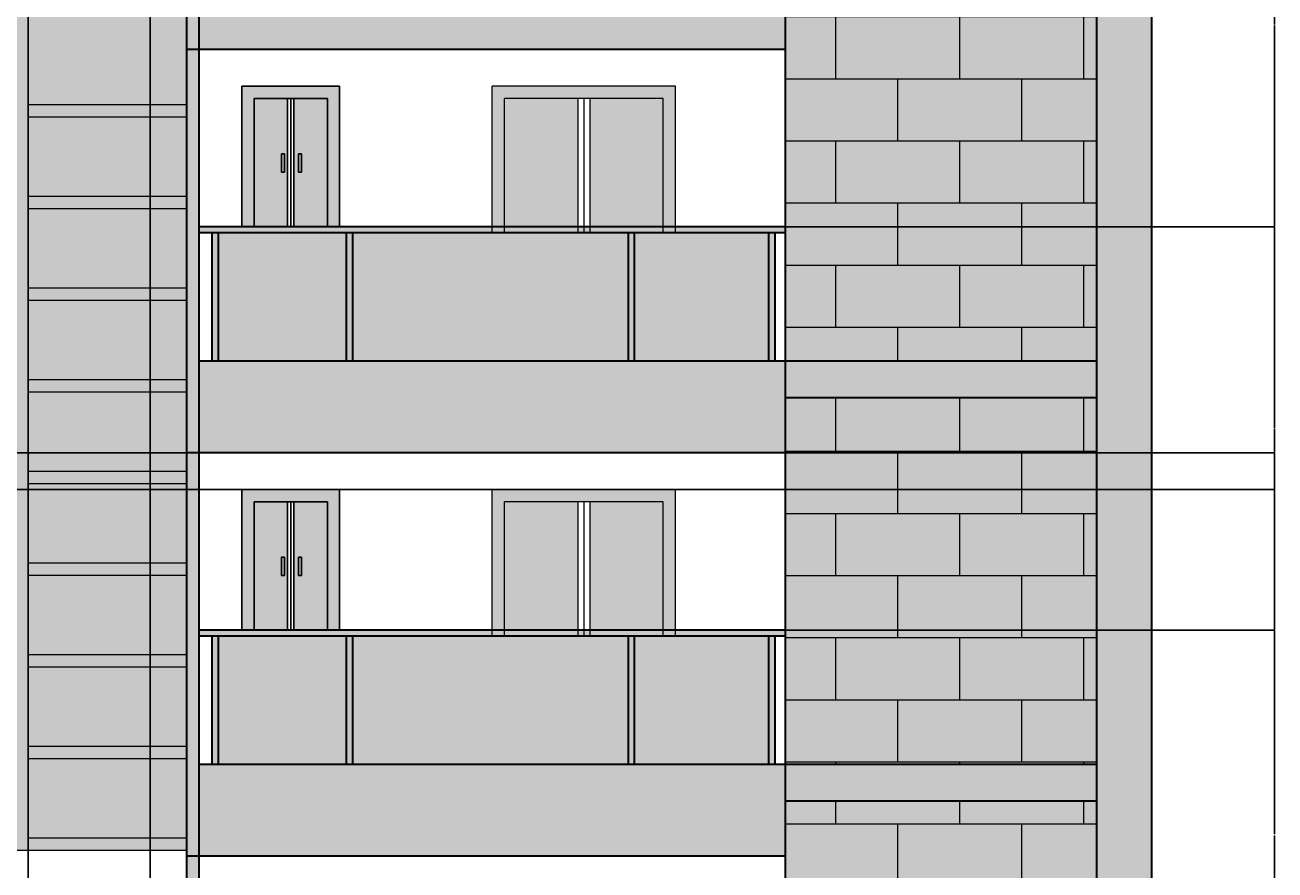
# Model space of a CAD drawing. Units: inches. Extents: x 2794 to 3619, y 522 to 1397.
# Tile 6 of 10: x 3209 to 3619, y 696 to 973. Entities that reach past the tile are written whole.
import ezdxf

# ---------------------------------------------------------------- set-up
doc = ezdxf.new("R2010")
doc.units = ezdxf.units.IN
for name, color, linetype, lineweight in [('A-ANNO-DIMS', 2, 'Continuous', 18), ('A-DOOR', 3, 'Continuous', 25), ('A-ELEV', 7, 'Continuous', 35), ('A-ELEV-PATT', 8, 'Continuous', 13), ('A-GLAZ', 4, 'Continuous', 18)]:
    doc.layers.add(name, color=color, linetype=linetype, lineweight=lineweight)
doc.styles.get("Standard").update_dxf_attribs({"font": 'arial.ttf'})
doc.dimstyles.get("Standard").update_dxf_attribs({"dimtxt": 0.18, "dimasz": 0.18, "dimexe": 0.18, "dimexo": 0.0625, "dimgap": 0.09, "dimtad": 0, "dimtih": 1, "dimtoh": 1, "dimdec": 4, "dimzin": 0, "dimdsep": 46, "dimtxsty": 'Standard', "dimcen": 0.09, "dimadec": 0, "dimazin": 0, "dimtfac": 1, "dimtdec": 4, "dimtofl": 0, "dimtmove": 0, "dimatfit": 3, "dimfxl": 1, "dimtolj": 1, "dimtzin": 0, "dimarcsym": 0})

# ---------------------------------------------------------------- blocks, each defined once
blk = doc.blocks.new('WIN-1500')
at = {"transparency": 33554646}
h = blk.add_hatch(color=256, dxfattribs=at)
h.dxf.hatch_style = 1
h.paths.add_polyline_path([(60, 48), (0, 48), (0, 2), (4, 2), (4, 44), (56, 44), (56, 2), (60, 2)])
at = {"transparency": 33554687}
h = blk.add_hatch(color=256, dxfattribs=at)
h.dxf.hatch_style = 1
h.set_gradient(color1=(248, 246, 176), color2=(74, 13, 14), name='INVCYLINDER')
h.paths.add_polyline_path([(56, 44), (32, 44), (32, 2), (56, 2)])
h.paths.add_polyline_path([(28, 44), (4, 44), (4, 2), (28, 2)])
for p, q in [((0, 0), (0, 48)), ((60, 48), (0, 48)), ((60, 0), (60, 48)), ((56, 44), (4, 44)), ((4, 0), (4, 44)), ((28, 44), (28, 0)), ((30, 44), (30, 0)), ((32, 44), (32, 0)), ((56, 0), (56, 44))]:
    blk.add_line(p, q)
blk = doc.blocks.new('DOOR-BALCONY-DBL')
at = {"transparency": 33554628}
h = blk.add_hatch(color=256, dxfattribs=at)
h.dxf.hatch_style = 1
h.paths.add_polyline_path([(4, 42), (28, 42), (28, 0), (32, 0), (32, 46), (0, 46), (0, 0), (4, 0)])
at = {"transparency": 33554646}
h = blk.add_hatch(color=256, dxfattribs=at)
h.dxf.hatch_style = 1
h.set_gradient(color1=(255, 255, 255), color2=(147, 149, 152), name='INVCYLINDER')
h.paths.add_polyline_path([(15, 42), (4, 42), (4, 0), (15, 0)])
h = blk.add_hatch(color=256, dxfattribs=at)
h.dxf.hatch_style = 1
h.set_gradient(color1=(255, 255, 255), color2=(147, 149, 152), name='INVCYLINDER')
h.paths.add_polyline_path([(28, 42), (17, 42), (17, 0), (28, 0)])
for p, q in [((0, 0), (0, 46)), ((0, 46), (32, 46)), ((4, 46), (28, 46)), ((32, 0), (32, 46)), ((4, 0), (4, 42)), ((4, 42), (28, 42)), ((15, 0), (15, 42)), ((16, 0), (16, 42)), ((17, 0), (17, 42)), ((28, 0), (28, 42))]:
    blk.add_line(p, q)
for points in [[(12.99, 23.83), (13.93, 23.83), (13.93, 17.87), (12.99, 17.87)], [(18.59, 23.83), (19.53, 23.83), (19.53, 17.87), (18.59, 17.87)]]:
    blk.add_lwpolyline(points, close=True)
blk = doc.blocks.new('*D19')
at = {"layer": 'A-ANNO-DIMS', "color": 0, "lineweight": -2, "transparency": 16777216}
for p, q in [((3458.33, 774.64), (3618.55, 774.64)), ((3618.37, 774.46), (3618.37, 707.82)), ((3618.37, 640.82), (3618.37, 707.45)), ((3458.33, 640.64), (3618.55, 640.64))]:
    blk.add_line(p, q, dxfattribs=at)
at = {"layer": 'A-ANNO-DIMS', "color": 0, "transparency": 16777216}
for points in [[(3618.34, 774.46), (3618.4, 774.46), (3618.37, 774.64)], [(3618.34, 640.82), (3618.4, 640.82), (3618.37, 640.64)]]:
    blk.add_solid(points, dxfattribs=at)
at = {"layer": 'Defpoints', "color": 0, "transparency": 16777216}
for p in [(3458.27, 774.64), (3618.37, 774.64), (3458.27, 640.64)]:
    blk.add_point(p, dxfattribs=at)
at = {"layer": 'A-ANNO-DIMS', "color": 0, "transparency": 16777216, "insert": (3618.37, 707.64), "char_height": 0.18, "attachment_point": 5}
blk.add_mtext('\\A1;134', dxfattribs=at)
blk = doc.blocks.new('*D20')
at = {"layer": 'A-ANNO-DIMS', "color": 0, "lineweight": -2, "transparency": 16777216}
for p, q in [((3458.33, 906.64), (3618.55, 906.64)), ((3618.37, 906.46), (3618.37, 840.82)), ((3618.37, 774.82), (3618.37, 840.45)), ((3458.33, 774.64), (3618.55, 774.64))]:
    blk.add_line(p, q, dxfattribs=at)
at = {"layer": 'A-ANNO-DIMS', "color": 0, "transparency": 16777216}
for points in [[(3618.34, 906.46), (3618.4, 906.46), (3618.37, 906.64)], [(3618.34, 774.82), (3618.4, 774.82), (3618.37, 774.64)]]:
    blk.add_solid(points, dxfattribs=at)
at = {"layer": 'Defpoints', "color": 0, "transparency": 16777216}
for p in [(3458.27, 906.64), (3618.37, 906.64), (3458.27, 774.64)]:
    blk.add_point(p, dxfattribs=at)
at = {"layer": 'A-ANNO-DIMS', "color": 0, "transparency": 16777216, "insert": (3618.37, 840.64), "char_height": 0.18, "attachment_point": 5}
blk.add_mtext('\\A1;132', dxfattribs=at)
blk = doc.blocks.new('*D21')
at = {"layer": 'A-ANNO-DIMS', "color": 0, "lineweight": -2, "transparency": 16777216}
for p, q in [((3458.33, 1038.64), (3618.55, 1038.64)), ((3618.37, 1038.46), (3618.37, 972.82)), ((3618.37, 906.82), (3618.37, 972.45)), ((3458.33, 906.64), (3618.55, 906.64))]:
    blk.add_line(p, q, dxfattribs=at)
at = {"layer": 'A-ANNO-DIMS', "color": 0, "transparency": 16777216}
for points in [[(3618.34, 1038.46), (3618.4, 1038.46), (3618.37, 1038.64)], [(3618.34, 906.82), (3618.4, 906.82), (3618.37, 906.64)]]:
    blk.add_solid(points, dxfattribs=at)
at = {"layer": 'Defpoints', "color": 0, "transparency": 16777216}
for p in [(3458.27, 1038.64), (3618.37, 1038.64), (3458.27, 906.64)]:
    blk.add_point(p, dxfattribs=at)
at = {"layer": 'A-ANNO-DIMS', "color": 0, "transparency": 16777216, "insert": (3618.37, 972.64), "char_height": 0.18, "attachment_point": 5}
blk.add_mtext('\\A1;132', dxfattribs=at)
blk = doc.blocks.new('*D43')
at = {"layer": 'A-ANNO-DIMS', "color": 0, "lineweight": -2, "transparency": 16777216}
for p, q in [((3150.33, 832.64), (3618.55, 832.64)), ((3618.37, 832.46), (3618.37, 826.82)), ((3618.37, 820.82), (3618.37, 826.45)), ((3132.33, 820.64), (3618.55, 820.64))]:
    blk.add_line(p, q, dxfattribs=at)
at = {"layer": 'A-ANNO-DIMS', "color": 0, "transparency": 16777216}
for points in [[(3618.34, 832.46), (3618.4, 832.46), (3618.37, 832.64)], [(3618.34, 820.82), (3618.4, 820.82), (3618.37, 820.64)]]:
    blk.add_solid(points, dxfattribs=at)
at = {"layer": 'Defpoints', "color": 0, "transparency": 16777216}
for p in [(3150.27, 832.64), (3618.37, 832.64), (3132.27, 820.64)]:
    blk.add_point(p, dxfattribs=at)
at = {"layer": 'A-ANNO-DIMS', "color": 0, "transparency": 16777216, "insert": (3618.37, 826.64), "char_height": 0.18, "attachment_point": 5}
blk.add_mtext('\\A1;12', dxfattribs=at)
blk = doc.blocks.new('*D51')
at = {"layer": 'A-ANNO-DIMS', "color": 0, "lineweight": -2, "transparency": 16777216}
for p, q in [((3206.27, 1254.57), (3206.27, 522.36)), ((3210.27, 1254.57), (3210.27, 522.36)), ((3206.45, 522.54), (3208.11, 522.54)), ((3210.09, 522.54), (3208.42, 522.54))]:
    blk.add_line(p, q, dxfattribs=at)
at = {"layer": 'A-ANNO-DIMS', "color": 0, "transparency": 16777216}
for points in [[(3206.45, 522.57), (3206.45, 522.51), (3206.27, 522.54)], [(3210.09, 522.57), (3210.09, 522.51), (3210.27, 522.54)]]:
    blk.add_solid(points, dxfattribs=at)
at = {"layer": 'Defpoints', "color": 0, "transparency": 16777216}
for p in [(3206.27, 1254.64), (3210.27, 1254.64), (3210.27, 522.54)]:
    blk.add_point(p, dxfattribs=at)
at = {"layer": 'A-ANNO-DIMS', "color": 0, "transparency": 16777216, "insert": (3208.27, 522.54), "char_height": 0.18, "attachment_point": 5}
blk.add_mtext('\\A1;4', dxfattribs=at)
blk = doc.blocks.new('*D52')
at = {"layer": 'A-ANNO-DIMS', "color": 0, "lineweight": -2, "transparency": 16777216}
for p, q in [((3210.27, 1254.57), (3210.27, 522.36)), ((3262.27, 1254.57), (3262.27, 522.36)), ((3210.45, 522.54), (3236.05, 522.54)), ((3262.09, 522.54), (3236.48, 522.54))]:
    blk.add_line(p, q, dxfattribs=at)
at = {"layer": 'A-ANNO-DIMS', "color": 0, "transparency": 16777216}
for points in [[(3210.45, 522.57), (3210.45, 522.51), (3210.27, 522.54)], [(3262.09, 522.57), (3262.09, 522.51), (3262.27, 522.54)]]:
    blk.add_solid(points, dxfattribs=at)
at = {"layer": 'Defpoints', "color": 0, "transparency": 16777216}
for p in [(3210.27, 1254.64), (3262.27, 1254.64), (3262.27, 522.54)]:
    blk.add_point(p, dxfattribs=at)
at = {"layer": 'A-ANNO-DIMS', "color": 0, "transparency": 16777216, "insert": (3236.27, 522.54), "char_height": 0.18, "attachment_point": 5}
blk.add_mtext('\\A1;52', dxfattribs=at)
blk = doc.blocks.new('*D56')
at = {"layer": 'A-ANNO-DIMS', "color": 0, "lineweight": -2, "transparency": 16777216}
for p, q in [((3162.27, 664.7), (3162.27, 1396.92)), ((3162.45, 1396.74), (3206.05, 1396.74)), ((3250.09, 1396.74), (3206.49, 1396.74)), ((3250.27, 664.7), (3250.27, 1396.92))]:
    blk.add_line(p, q, dxfattribs=at)
at = {"layer": 'A-ANNO-DIMS', "color": 0, "transparency": 16777216}
for points in [[(3162.45, 1396.77), (3162.45, 1396.71), (3162.27, 1396.74)], [(3250.09, 1396.77), (3250.09, 1396.71), (3250.27, 1396.74)]]:
    blk.add_solid(points, dxfattribs=at)
at = {"layer": 'Defpoints', "color": 0, "transparency": 16777216}
for p in [(3250.27, 1396.74), (3162.27, 664.64), (3250.27, 664.64)]:
    blk.add_point(p, dxfattribs=at)
at = {"layer": 'A-ANNO-DIMS', "color": 0, "transparency": 16777216, "insert": (3206.27, 1396.74), "char_height": 0.18, "attachment_point": 5}
blk.add_mtext('\\A1;88', dxfattribs=at)

msp = doc.modelspace()

# ---------------------------------------------------------------- hatches: boundary and pattern name
at = {"layer": 'A-ELEV-PATT', "transparency": 33554687}
h = msp.add_hatch(color=256, dxfattribs=at)
h.dxf.hatch_style = 1
h.paths.add_polyline_path([(3262.2659, 1350.6351), (3150.2659, 1350.6351), (3150.2659, 1279.0155, -0.68639605), (3262.2659, 1279.0155)])
h.paths.add_polyline_path([(3210.2659, 1314.1121), (3210.2659, 1258.6351), (3262.2659, 1258.6351, 0.39146256)])
h.paths.add_polyline_path([(3206.2659, 1314.2551, 0.41222069), (3150.2659, 1258.6351), (3206.2659, 1258.6351)])
h.paths.add_polyline_path([(3262.2659, 1254.6351), (3210.2659, 1254.6351), (3210.2659, 1216.6351), (3262.2659, 1216.6351)])
h.paths.add_polyline_path([(3206.2659, 1254.6351), (3150.2659, 1254.6351), (3150.2659, 1216.6351), (3206.2659, 1216.6351)])
h.paths.add_polyline_path([(3262.2659, 1212.6351), (3210.2659, 1212.6351), (3210.2659, 1186.6351), (3262.2659, 1186.6351)])
h.paths.add_polyline_path([(3206.2659, 1212.6351), (3150.2659, 1212.6351), (3150.2659, 1186.6351), (3206.2659, 1186.6351)])
h.paths.add_polyline_path([(3206.2659, 1182.6351), (3150.2659, 1182.6351), (3150.2659, 1156.6351), (3206.2659, 1156.6351)])
h.paths.add_polyline_path([(3262.2659, 1182.6351), (3210.2659, 1182.6351), (3210.2659, 1156.6351), (3262.2659, 1156.6351)])
h.paths.add_polyline_path([(3262.2659, 1152.6351), (3210.2659, 1152.6351), (3210.2659, 1126.6351), (3262.2659, 1126.6351)])
h.paths.add_polyline_path([(3206.2659, 1152.6351), (3150.2659, 1152.6351), (3150.2659, 1126.6351), (3206.2659, 1126.6351)])
h.paths.add_polyline_path([(3262.2659, 1122.6351), (3210.2659, 1122.6351), (3210.2659, 1096.6351), (3262.2659, 1096.6351)])
h.paths.add_polyline_path([(3206.2659, 1122.6351), (3150.2659, 1122.6351), (3150.2659, 1096.6351), (3206.2659, 1096.6351)])
h.paths.add_polyline_path([(3206.2659, 1092.6351), (3150.2659, 1092.6351), (3150.2659, 1066.6351), (3206.2659, 1066.6351)])
h.paths.add_polyline_path([(3262.2659, 1092.6351), (3210.2659, 1092.6351), (3210.2659, 1066.6351), (3262.2659, 1066.6351)])
h.paths.add_polyline_path([(3262.2659, 1062.6351), (3210.2659, 1062.6351), (3210.2659, 1036.6351), (3262.2659, 1036.6351)])
h.paths.add_polyline_path([(3206.2659, 1062.6351), (3150.2659, 1062.6351), (3150.2659, 1036.6351), (3206.2659, 1036.6351)])
h.paths.add_polyline_path([(3206.2659, 1032.6351), (3150.2659, 1032.6351), (3150.2659, 1006.6351), (3206.2659, 1006.6351)])
h.paths.add_polyline_path([(3262.2659, 1032.6351), (3210.2659, 1032.6351), (3210.2659, 1006.6351), (3262.2659, 1006.6351)])
h.paths.add_polyline_path([(3262.2659, 1002.6351), (3210.2659, 1002.6351), (3210.2659, 976.6351), (3262.2659, 976.6351)])
h.paths.add_polyline_path([(3206.2659, 1002.6351), (3150.2659, 1002.6351), (3150.2659, 976.6351), (3206.2659, 976.6351)])
h.paths.add_polyline_path([(3206.2659, 972.6351), (3150.2659, 972.6351), (3150.2659, 946.6351), (3206.2659, 946.6351)])
h.paths.add_polyline_path([(3206.2659, 942.6351), (3150.2659, 942.6351), (3150.2659, 916.6351), (3206.2659, 916.6351)])
h.paths.add_polyline_path([(3262.2659, 942.6351), (3210.2659, 942.6351), (3210.2659, 916.6351), (3262.2659, 916.6351)])
h.paths.add_polyline_path([(3262.2659, 972.6351), (3210.2659, 972.6351), (3210.2659, 946.6351), (3262.2659, 946.6351)])
h.paths.add_polyline_path([(3262.2659, 912.6351), (3210.2659, 912.6351), (3210.2659, 886.6351), (3262.2659, 886.6351)])
h.paths.add_polyline_path([(3206.2659, 912.6351), (3150.2659, 912.6351), (3150.2659, 886.6351), (3206.2659, 886.6351)])
h.paths.add_polyline_path([(3206.2659, 882.6351), (3150.2659, 882.6351), (3150.2659, 856.6351), (3206.2659, 856.6351)])
h.paths.add_polyline_path([(3262.2659, 882.6351), (3210.2659, 882.6351), (3210.2659, 856.6351), (3262.2659, 856.6351)])
h.paths.add_polyline_path([(3262.2659, 852.6351), (3210.2659, 852.6351), (3210.2659, 826.6351), (3262.2659, 826.6351)])
h.paths.add_polyline_path([(3206.2659, 852.6351), (3150.2659, 852.6351), (3150.2659, 826.6351), (3206.2659, 826.6351)])
h.paths.add_polyline_path([(3206.2659, 822.6351), (3150.2659, 822.6351), (3150.2659, 796.6351), (3206.2659, 796.6351)])
h.paths.add_polyline_path([(3262.2659, 822.6351), (3210.2659, 822.6351), (3210.2659, 796.6351), (3262.2659, 796.6351)])
h.paths.add_polyline_path([(3262.2659, 792.6351), (3210.2659, 792.6351), (3210.2659, 766.6351), (3262.2659, 766.6351)])
h.paths.add_polyline_path([(3206.2659, 792.6351), (3150.2659, 792.6351), (3150.2659, 766.6351), (3206.2659, 766.6351)])
h.paths.add_polyline_path([(3206.2659, 762.6351), (3150.2659, 762.6351), (3150.2659, 736.6351), (3206.2659, 736.6351)])
h.paths.add_polyline_path([(3206.2659, 732.6351), (3150.2659, 732.6351), (3150.2659, 706.6351), (3206.2659, 706.6351)])
h.paths.add_polyline_path([(3262.2659, 732.6351), (3210.2659, 732.6351), (3210.2659, 706.6351), (3262.2659, 706.6351)])
h.paths.add_polyline_path([(3262.2659, 762.6351), (3210.2659, 762.6351), (3210.2659, 736.6351), (3262.2659, 736.6351)])
h = msp.add_hatch(color=256, dxfattribs=at)
h.dxf.hatch_style = 1
h.paths.add_polyline_path([(3150.2659, 1257.8725, -0.00340445), (3150.2659, 1258.6351), (3146.2659, 1258.6351), (3146.2659, 1228.6351), (3150.2659, 1228.6351)])
h.paths.add_polyline_path([(3262.2659, 1258.6351), (3210.2659, 1258.6351), (3210.2659, 1314.1121, 0.01787385), (3206.2659, 1314.2551), (3206.2659, 1258.6351), (3150.2659, 1258.6351), (3150.2659, 1254.6351), (3206.2659, 1254.6351), (3206.2659, 1216.6351), (3150.2659, 1216.6351), (3150.2659, 1212.6351), (3206.2659, 1212.6351), (3206.2659, 1186.6351), (3150.2659, 1186.6351), (3150.2659, 1182.6351), (3206.2659, 1182.6351), (3206.2659, 1156.6351), (3150.2659, 1156.6351), (3150.2659, 1152.6351), (3206.2659, 1152.6351), (3206.2659, 1126.6351), (3150.2659, 1126.6351), (3150.2659, 1122.6351), (3206.2659, 1122.6351), (3206.2659, 1096.6351), (3150.2659, 1096.6351), (3150.2659, 1092.6351), (3206.2659, 1092.6351), (3206.2659, 1066.6351), (3150.2659, 1066.6351), (3150.2659, 1062.6351), (3206.2659, 1062.6351), (3206.2659, 1036.6351), (3150.2659, 1036.6351), (3150.2659, 1032.6351), (3206.2659, 1032.6351), (3206.2659, 1006.6351), (3150.2659, 1006.6351), (3150.2659, 1002.6351), (3206.2659, 1002.6351), (3206.2659, 976.6351), (3150.2659, 976.6351), (3150.2659, 972.6351), (3206.2659, 972.6351), (3206.2659, 946.6351), (3150.2659, 946.6351), (3150.2659, 942.6351), (3206.2659, 942.6351), (3206.2659, 916.6351), (3150.2659, 916.6351), (3150.2659, 912.6351), (3206.2659, 912.6351), (3206.2659, 886.6351), (3150.2659, 886.6351), (3150.2659, 882.6351), (3206.2659, 882.6351), (3206.2659, 856.6351), (3150.2659, 856.6351), (3150.2659, 852.6351), (3206.2659, 852.6351), (3206.2659, 826.6351), (3150.2659, 826.6351), (3150.2659, 822.6351), (3206.2659, 822.6351), (3206.2659, 796.6351), (3150.2659, 796.6351), (3150.2659, 792.6351), (3206.2659, 792.6351), (3206.2659, 766.6351), (3150.2659, 766.6351), (3150.2659, 762.6351), (3206.2659, 762.6351), (3206.2659, 736.6351), (3150.2659, 736.6351), (3150.2659, 732.6351), (3206.2659, 732.6351), (3206.2659, 706.6351), (3150.2659, 706.6351), (3150.2659, 702.6351), (3262.2659, 702.6351), (3262.2659, 706.6351), (3210.2659, 706.6351), (3210.2659, 732.6351), (3262.2659, 732.6351), (3262.2659, 736.6351), (3210.2659, 736.6351), (3210.2659, 762.6351), (3262.2659, 762.6351), (3262.2659, 766.6351), (3210.2659, 766.6351), (3210.2659, 792.6351), (3262.2659, 792.6351), (3262.2659, 796.6351), (3210.2659, 796.6351), (3210.2659, 822.6351), (3262.2659, 822.6351), (3262.2659, 826.6351), (3210.2659, 826.6351), (3210.2659, 852.6351), (3262.2659, 852.6351), (3262.2659, 856.6351), (3210.2659, 856.6351), (3210.2659, 882.6351), (3262.2659, 882.6351), (3262.2659, 886.6351), (3210.2659, 886.6351), (3210.2659, 912.6351), (3262.2659, 912.6351), (3262.2659, 916.6351), (3210.2659, 916.6351), (3210.2659, 942.6351), (3262.2659, 942.6351), (3262.2659, 946.6351), (3210.2659, 946.6351), (3210.2659, 972.6351), (3262.2659, 972.6351), (3262.2659, 976.6351), (3210.2659, 976.6351), (3210.2659, 1002.6351), (3262.2659, 1002.6351), (3262.2659, 1006.6351), (3210.2659, 1006.6351), (3210.2659, 1032.6351), (3262.2659, 1032.6351), (3262.2659, 1036.6351), (3210.2659, 1036.6351), (3210.2659, 1062.6351), (3262.2659, 1062.6351), (3262.2659, 1066.6351), (3210.2659, 1066.6351), (3210.2659, 1092.6351), (3262.2659, 1092.6351), (3262.2659, 1096.6351), (3210.2659, 1096.6351), (3210.2659, 1122.6351), (3262.2659, 1122.6351), (3262.2659, 1126.6351), (3210.2659, 1126.6351), (3210.2659, 1152.6351), (3262.2659, 1152.6351), (3262.2659, 1156.6351), (3210.2659, 1156.6351), (3210.2659, 1182.6351), (3262.2659, 1182.6351), (3262.2659, 1186.6351), (3210.2659, 1186.6351), (3210.2659, 1212.6351), (3262.2659, 1212.6351), (3262.2659, 1216.6351), (3210.2659, 1216.6351), (3210.2659, 1254.6351), (3262.2659, 1254.6351)])
h = msp.add_hatch(color=256, dxfattribs=at)
h.dxf.hatch_style = 1
h.paths.add_polyline_path([(3578.2659, 1294.6351), (3560.2659, 1294.6351), (3560.2659, 642.6351), (3578.2659, 642.6351)])
h.paths.add_polyline_path([(2852.2659, 1294.6351), (2834.2659, 1294.6351), (2834.2659, 642.6351), (2852.2659, 642.6351)])
h = msp.add_hatch(color=256, dxfattribs=at)
h.dxf.hatch_style = 1
h.paths.add_polyline_path([(2852.2659, 1294.6351), (2834.2659, 1294.6351), (2834.2659, 562.6351), (2852.2659, 562.6351)])
h.paths.add_polyline_path([(3578.2659, 1294.6351), (3560.2659, 1294.6351), (3560.2659, 562.6351), (3578.2659, 562.6351)])
h = msp.add_hatch(color=256, dxfattribs=at)
h.dxf.hatch_style = 1
h.paths.add_polyline_path([(2852.2659, 1246.6351), (2954.2659, 1246.6351), (2954.2659, 1258.6351), (2900.2659, 1258.6351), (2900.2659, 1294.6351), (2852.2659, 1294.6351)])
h.paths.add_polyline_path([(3512.2659, 1294.6351), (3512.2659, 1258.6351), (3458.2659, 1258.6351), (3458.2659, 1246.6351), (3560.2659, 1246.6351), (3560.2659, 1294.6351)])
h.paths.add_polyline_path([(2954.2659, 1114.6351), (2954.2659, 1126.6351), (2852.2659, 1126.6351), (2852.2659, 1114.6351)])
h.paths.add_polyline_path([(3560.2659, 1114.6351), (3560.2659, 1126.6351), (3458.2659, 1126.6351), (3458.2659, 1114.6351)])
h.paths.add_polyline_path([(3560.2659, 982.6351), (3560.2659, 994.6351), (3458.2659, 994.6351), (3458.2659, 982.6351)])
h.paths.add_polyline_path([(2954.2659, 982.6351), (2954.2659, 994.6351), (2852.2659, 994.6351), (2852.2659, 982.6351)])
h.paths.add_polyline_path([(2852.2659, 862.6351), (2852.2659, 850.6351), (2954.2659, 850.6351), (2954.2659, 862.6351)])
h.paths.add_polyline_path([(2852.2659, 730.6351), (2852.2659, 718.6351), (2954.2659, 718.6351), (2954.2659, 730.6351)])
h.paths.add_polyline_path([(3560.2659, 718.6351), (3560.2659, 730.6351), (3458.2659, 730.6351), (3458.2659, 718.6351)])
h.paths.add_polyline_path([(3560.2659, 850.6351), (3560.2659, 862.6351), (3458.2659, 862.6351), (3458.2659, 850.6351)])
h = msp.add_hatch(color=256, dxfattribs=at)
h.dxf.hatch_style = 1
h.paths.add_polyline_path([(3146.2659, 1096.6351), (3146.2659, 1126.6351), (2954.2659, 1126.6351), (2954.2659, 1096.6351)])
h.paths.add_polyline_path([(3458.2659, 1096.6351), (3458.2659, 1126.6351), (3266.2659, 1126.6351), (3266.2659, 1096.6351)])
h.paths.add_polyline_path([(3458.2659, 964.6351), (3458.2659, 994.6351), (3266.2659, 994.6351), (3266.2659, 964.6351)])
h.paths.add_polyline_path([(3146.2659, 964.6351), (3146.2659, 994.6351), (2954.2659, 994.6351), (2954.2659, 964.6351)])
h.paths.add_polyline_path([(3458.2659, 832.6351), (3458.2659, 862.6351), (3266.2659, 862.6351), (3266.2659, 832.6351)])
h.paths.add_polyline_path([(3146.2659, 832.6351), (3146.2659, 862.6351), (2954.2659, 862.6351), (2954.2659, 832.6351)])
h.paths.add_polyline_path([(3458.2659, 700.6351), (3458.2659, 730.6351), (3266.2659, 730.6351), (3266.2659, 700.6351)])
h.paths.add_polyline_path([(3146.2659, 700.6351), (3146.2659, 730.6351), (2954.2659, 730.6351), (2954.2659, 700.6351)])
h.paths.add_polyline_path([(3266.2659, 1294.6351), (3266.2659, 1258.6351), (3266.2659, 1228.6351), (3458.2659, 1228.6351), (3458.2659, 1294.6351)])
h.paths.add_polyline_path([(3146.2659, 1228.6351), (3146.2659, 1256.2485, -0.00994307), (3146.2659, 1258.6351), (3146.2659, 1294.6351), (2954.2659, 1294.6351), (2954.2659, 1228.6351)])
at = {"layer": 'A-ELEV-PATT'}
h = msp.add_hatch(dxfattribs=at)
h.set_pattern_fill('AR-B816', color=256, scale=0.1)
h.paths.add_polyline_path([(2954.2659, 1114.6351), (2852.2659, 1114.6351), (2852.2659, 994.6351), (2954.2659, 994.6351)])
h.paths.add_polyline_path([(2954.2659, 1246.6351), (2852.2659, 1246.6351), (2852.2659, 1126.6351), (2954.2659, 1126.6351)])
h.paths.add_polyline_path([(2954.2659, 982.6351), (2852.2659, 982.6351), (2852.2659, 862.6351), (2954.2659, 862.6351)])
h.paths.add_polyline_path([(2954.2659, 850.6351), (2852.2659, 850.6351), (2852.2659, 730.6351), (2954.2659, 730.6351)])
h.paths.add_polyline_path([(3560.2659, 850.6351), (3458.2659, 850.6351), (3458.2659, 730.6351), (3560.2659, 730.6351)])
h.paths.add_polyline_path([(3560.2659, 982.6351), (3458.2659, 982.6351), (3458.2659, 862.6351), (3560.2659, 862.6351)])
h.paths.add_polyline_path([(3560.2659, 1114.6351), (3458.2659, 1114.6351), (3458.2659, 994.6351), (3560.2659, 994.6351)])
h.paths.add_polyline_path([(3560.2659, 1246.6351), (3458.2659, 1246.6351), (3458.2659, 1126.6351), (3560.2659, 1126.6351)])
h.paths.add_polyline_path([(2852.2659, 642.6351), (2954.2659, 642.6351), (2954.2659, 718.6351), (2852.2659, 718.6351)])
h.paths.add_polyline_path([(3458.2659, 640.6351), (3560.2659, 640.6351), (3560.2659, 718.6351), (3458.2659, 718.6351)])
at = {"layer": 'A-ELEV-PATT', "transparency": 33554630}
h = msp.add_hatch(color=256, dxfattribs=at)
h.dxf.hatch_style = 1
h.paths.add_polyline_path([(2954.2659, 1114.6351), (2852.2659, 1114.6351), (2852.2659, 994.6351), (2954.2659, 994.6351)])
h.paths.add_polyline_path([(2954.2659, 982.6351), (2852.2659, 982.6351), (2852.2659, 862.6351), (2954.2659, 862.6351)])
h.paths.add_polyline_path([(2954.2659, 850.6351), (2852.2659, 850.6351), (2852.2659, 730.6351), (2954.2659, 730.6351)])
h.paths.add_polyline_path([(3560.2659, 850.6351), (3458.2659, 850.6351), (3458.2659, 730.6351), (3560.2659, 730.6351)])
h.paths.add_polyline_path([(3560.2659, 982.6351), (3458.2659, 982.6351), (3458.2659, 862.6351), (3560.2659, 862.6351)])
h.paths.add_polyline_path([(3560.2659, 1114.6351), (3458.2659, 1114.6351), (3458.2659, 994.6351), (3560.2659, 994.6351)])
h.paths.add_polyline_path([(3560.2659, 1246.6351), (3458.2659, 1246.6351), (3458.2659, 1126.6351), (3560.2659, 1126.6351)])
h.paths.add_polyline_path([(2852.2659, 642.6351), (2954.2659, 642.6351), (2954.2659, 718.6351), (2852.2659, 718.6351)])
h.paths.add_polyline_path([(3458.2659, 642.6351), (3560.2659, 642.6351), (3560.2659, 718.6351), (3458.2659, 718.6351)])
at = {"layer": 'A-ELEV-PATT', "transparency": 33554687}
h = msp.add_hatch(color=256, dxfattribs=at)
h.dxf.hatch_style = 1
h.paths.add_polyline_path([(3262.2659, 964.6351), (3266.2659, 964.6351), (3266.2659, 1038.6351), (3262.2659, 1038.6351)])
h = msp.add_hatch(color=256, dxfattribs=at)
h.dxf.hatch_style = 1
h.paths.add_polyline_path([(3266.2659, 964.6351), (3262.2659, 964.6351), (3262.2659, 832.6351), (3266.2659, 832.6351)])
h = msp.add_hatch(color=256, dxfattribs=at)
h.dxf.hatch_style = 1
h.paths.add_polyline_path([(3316.4761, 904.6351), (3314.4761, 904.6351), (3314.4761, 862.6351), (3316.4761, 862.6351)])
h.paths.add_polyline_path([(3272.4761, 904.6351), (3270.4761, 904.6351), (3270.4761, 862.6351), (3272.4761, 862.6351)])
h.paths.add_polyline_path([(3458.2659, 906.6351), (3266.2659, 906.6351), (3266.2659, 904.6351), (3458.2659, 904.6351)])
h.paths.add_polyline_path([(3408.7822, 904.6351), (3406.7822, 904.6351), (3406.7822, 862.6351), (3408.7822, 862.6351)])
h.paths.add_polyline_path([(3454.7613, 904.6351), (3452.7613, 904.6351), (3452.7613, 862.6351), (3454.7613, 862.6351)])
h = msp.add_hatch(color=256, dxfattribs=at)
h.dxf.hatch_style = 1
h.paths.add_polyline_path([(3262.2659, 700.6351), (3266.2659, 700.6351), (3266.2659, 832.6351), (3262.2659, 832.6351)])
h = msp.add_hatch(color=256, dxfattribs=at)
h.dxf.hatch_style = 1
h.paths.add_polyline_path([(3458.2659, 774.6351), (3266.2659, 774.6351), (3266.2659, 772.6351), (3458.2659, 772.6351)])
h.paths.add_polyline_path([(3316.4761, 772.6351), (3314.4761, 772.6351), (3314.4761, 730.6351), (3316.4761, 730.6351)])
h.paths.add_polyline_path([(3272.4761, 772.6351), (3270.4761, 772.6351), (3270.4761, 730.6351), (3272.4761, 730.6351)])
h.paths.add_polyline_path([(3408.7822, 772.6351), (3406.7822, 772.6351), (3406.7822, 730.6351), (3408.7822, 730.6351)])
h.paths.add_polyline_path([(3454.7613, 772.6351), (3452.7613, 772.6351), (3452.7613, 730.6351), (3454.7613, 730.6351)])
h = msp.add_hatch(color=256, dxfattribs=at)
h.dxf.hatch_style = 1
h.paths.add_polyline_path([(3266.2659, 700.6351), (3262.2659, 700.6351), (3262.2659, 642.6351), (3266.2659, 642.6351)])
h.paths.add_polyline_path([(3266.2659, 640.6351), (3262.2659, 640.6351), (3262.2659, 598.6351), (3266.2659, 598.6351)])
h.paths.add_polyline_path([(3458.2659, 642.6351), (3266.2659, 642.6351), (3266.2659, 640.6351), (3458.2659, 640.6351)])
h.paths.add_polyline_path([(3272.4761, 640.6351), (3270.4761, 640.6351), (3270.4761, 598.6351), (3272.4761, 598.6351)])
h.paths.add_polyline_path([(3316.4761, 640.6351), (3314.4761, 640.6351), (3314.4761, 598.6351), (3316.4761, 598.6351)])
h.paths.add_polyline_path([(3266.2659, 642.6351), (3262.2659, 642.6351), (3262.2659, 640.6351), (3266.2659, 640.6351)])
h.paths.add_polyline_path([(3150.2659, 640.6351), (3146.2659, 640.6351), (3146.2659, 598.6351), (3150.2659, 598.6351)])
at = {"layer": 'A-GLAZ', "transparency": 33554556}
h = msp.add_hatch(color=256, dxfattribs=at)
h.dxf.hatch_style = 1
h.set_gradient(color1=(255, 255, 255), color2=(0, 255, 255), name='INVCYLINDER')
h.paths.add_polyline_path([(3314.4761, 904.6351), (3272.4761, 904.6351), (3272.4761, 862.6351), (3314.4761, 862.6351)])
h.paths.add_polyline_path([(3452.7613, 904.6351), (3408.7822, 904.6351), (3408.7822, 862.6351), (3452.7613, 862.6351)])
h = msp.add_hatch(color=256, dxfattribs=at)
h.dxf.hatch_style = 1
h.set_gradient(color1=(255, 255, 255), color2=(0, 255, 255), name='INVCYLINDER')
h.paths.add_polyline_path([(3406.7822, 904.6351), (3316.4761, 904.6351), (3316.4761, 862.6351), (3406.7822, 862.6351)])
h = msp.add_hatch(color=256, dxfattribs=at)
h.dxf.hatch_style = 1
h.set_gradient(color1=(255, 255, 255), color2=(0, 255, 255), name='INVCYLINDER')
h.paths.add_polyline_path([(3314.4761, 772.6351), (3272.4761, 772.6351), (3272.4761, 730.6351), (3314.4761, 730.6351)])
h = msp.add_hatch(color=256, dxfattribs=at)
h.dxf.hatch_style = 1
h.set_gradient(color1=(255, 255, 255), color2=(0, 255, 255), name='INVCYLINDER')
h.paths.add_polyline_path([(3406.7822, 772.6351), (3316.4761, 772.6351), (3316.4761, 730.6351), (3406.7822, 730.6351)])
h = msp.add_hatch(color=256, dxfattribs=at)
h.dxf.hatch_style = 1
h.set_gradient(color1=(255, 255, 255), color2=(0, 255, 255), name='INVCYLINDER')
h.paths.add_polyline_path([(3452.7613, 772.6351), (3408.7822, 772.6351), (3408.7822, 730.6351), (3452.7613, 730.6351)])

# ---------------------------------------------------------------- linework, layer by layer
at = {"layer": 'A-ELEV'}
for p, q in [((3578.2659, 562.6351), (3578.2659, 1297.6351)), ((3458.2659, 598.6351), (3458.2659, 1294.6351)), ((3560.2659, 562.6351), (3560.2659, 1294.6351)), ((3262.2659, 598.6351), (3262.2659, 1258.6351)), ((3266.2659, 598.6351), (3266.2659, 1258.6351)), ((3458.2659, 964.6351), (3262.2659, 964.6351)), ((3458.2659, 906.6351), (3266.2659, 906.6351)), ((3458.2659, 904.6351), (3266.2659, 904.6351)), ((3270.4761, 904.6351), (3270.4761, 862.6351)), ((3272.4761, 904.6351), (3272.4761, 862.6351)), ((3314.4761, 904.6351), (3314.4761, 862.6351)), ((3316.4761, 904.6351), (3316.4761, 862.6351)), ((3406.7822, 904.6351), (3406.7822, 862.6351)), ((3408.7822, 904.6351), (3408.7822, 862.6351)), ((3452.7613, 904.6351), (3452.7613, 862.6351)), ((3454.7613, 904.6351), (3454.7613, 862.6351)), ((3560.2659, 862.6351), (3266.2659, 862.6351)), ((3560.2659, 850.6351), (3458.2659, 850.6351)), ((3458.2659, 832.6351), (3262.2659, 832.6351)), ((3458.2659, 774.6351), (3266.2659, 774.6351)), ((3458.2659, 772.6351), (3266.2659, 772.6351)), ((3270.4761, 772.6351), (3270.4761, 730.6351)), ((3272.4761, 772.6351), (3272.4761, 730.6351)), ((3314.4761, 772.6351), (3314.4761, 730.6351)), ((3316.4761, 772.6351), (3316.4761, 730.6351)), ((3406.7822, 772.6351), (3406.7822, 730.6351)), ((3408.7822, 772.6351), (3408.7822, 730.6351)), ((3452.7613, 772.6351), (3452.7613, 730.6351)), ((3454.7613, 772.6351), (3454.7613, 730.6351)), ((3560.2659, 730.6351), (3266.2659, 730.6351)), ((3560.2659, 718.6351), (3458.2659, 718.6351)), ((3458.2659, 700.6351), (3262.2659, 700.6351))]:
    msp.add_line(p, q, dxfattribs=at)
at = {"layer": 'A-GLAZ'}
for p, q in [((3210.2659, 972.6351), (3210.2659, 946.6351)), ((3210.2659, 946.6351), (3262.2659, 946.6351)), ((3210.2659, 942.6351), (3210.2659, 916.6351)), ((3210.2659, 942.6351), (3262.2659, 942.6351)), ((3210.2659, 916.6351), (3262.2659, 916.6351)), ((3210.2659, 912.6351), (3210.2659, 886.6351)), ((3210.2659, 912.6351), (3262.2659, 912.6351)), ((3210.2659, 886.6351), (3262.2659, 886.6351)), ((3210.2659, 882.6351), (3210.2659, 856.6351)), ((3210.2659, 882.6351), (3262.2659, 882.6351)), ((3210.2659, 856.6351), (3262.2659, 856.6351)), ((3210.2659, 852.6351), (3210.2659, 826.6351)), ((3210.2659, 852.6351), (3262.2659, 852.6351)), ((3210.2659, 826.6351), (3262.2659, 826.6351)), ((3210.2659, 822.6351), (3210.2659, 796.6351)), ((3210.2659, 822.6351), (3262.2659, 822.6351)), ((3210.2659, 796.6351), (3262.2659, 796.6351)), ((3210.2659, 792.6351), (3210.2659, 766.6351)), ((3210.2659, 792.6351), (3262.2659, 792.6351)), ((3210.2659, 766.6351), (3262.2659, 766.6351)), ((3210.2659, 762.6351), (3210.2659, 736.6351)), ((3210.2659, 762.6351), (3262.2659, 762.6351)), ((3210.2659, 736.6351), (3262.2659, 736.6351)), ((3210.2659, 732.6351), (3210.2659, 706.6351)), ((3210.2659, 732.6351), (3262.2659, 732.6351)), ((3210.2659, 706.6351), (3262.2659, 706.6351)), ((3150.2659, 702.6351), (3262.2659, 702.6351))]:
    msp.add_line(p, q, dxfattribs=at)

# ---------------------------------------------------------------- block references
at = {"layer": 'A-DOOR'}
for p in [(3280.266, 906.635), (3280.266, 774.635)]:
    msp.add_blockref('DOOR-BALCONY-DBL', p, dxfattribs=at)
at = {"layer": 'A-GLAZ'}
for p in [(3362.266, 904.635), (3362.266, 772.635)]:
    msp.add_blockref('WIN-1500', p, dxfattribs=at)

# ---------------------------------------------------------------- dimensions: what is measured, and where the dimension line sits
at = {"layer": 'A-ANNO-DIMS'}
for base, p1, p2, picture, middle in [((3250.2659, 1396.7351), (3162.2659, 664.6351), (3250.2659, 664.6351), '*D56', (3206.2659, 1396.7351)), ((3210.2659, 522.5351), (3206.2659, 1254.6351), (3210.2659, 1254.6351), '*D51', (3208.2659, 522.5351)), ((3262.2659, 522.5351), (3210.2659, 1254.6351), (3262.2659, 1254.6351), '*D52', (3236.2659, 522.5351))]:
    dim = msp.add_linear_dim(base=base, p1=p1, p2=p2, dimstyle='Standard', override={"dimdec": 0, "dimlfac": 1, "dimrnd": 0, "dimzin": 0, "dimdsep": 46, "dimlunit": 2}, dxfattribs=at)
    dim.commit()
    dim.dimension.update_dxf_attribs({"geometry": picture, "text_midpoint": middle})
for base, p1, p2, picture, middle in [((3618.3659, 1038.6351), (3458.2659, 906.6351), (3458.2659, 1038.6351), '*D21', (3618.3659, 972.6351)), ((3618.3659, 906.6351), (3458.2659, 774.6351), (3458.2659, 906.6351), '*D20', (3618.3659, 840.6351)), ((3618.3659, 832.6351), (3132.2659, 820.6351), (3150.2659, 832.6351), '*D43', (3618.3659, 826.6351)), ((3618.3659, 774.6351), (3458.2659, 640.6351), (3458.2659, 774.6351), '*D19', (3618.3659, 707.6351))]:
    dim = msp.add_linear_dim(base=base, p1=p1, p2=p2, angle=90, dimstyle='Standard', override={"dimdec": 0, "dimlfac": 1, "dimrnd": 0, "dimzin": 0, "dimdsep": 46, "dimlunit": 2}, dxfattribs=at)
    dim.commit()
    dim.dimension.update_dxf_attribs({"geometry": picture, "text_midpoint": middle})

doc.saveas('drawing.dxf')
